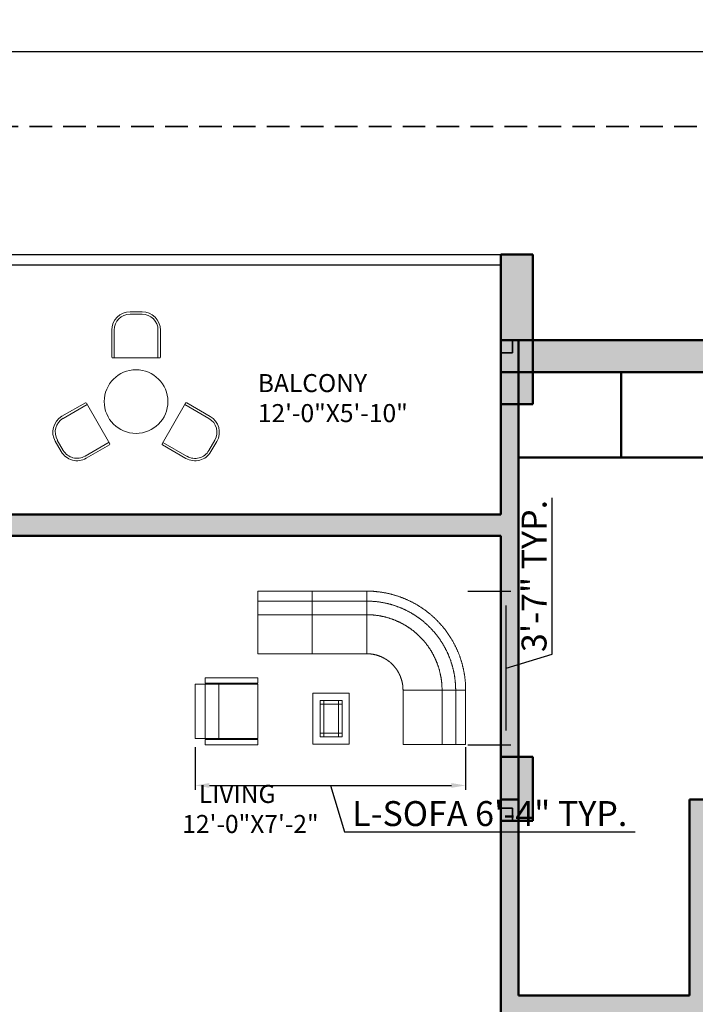
# Model space of a CAD drawing. Units: inches. Extents: x -7 to 1228, y -146 to 1091.
# Tile 87 of 88: x 816 to 1006, y 814 to 1091. Entities that reach past the tile are written whole.
import ezdxf

# ---------------------------------------------------------------- set-up
doc = ezdxf.new("R2010")
doc.units = ezdxf.units.IN
doc.linetypes.add('DASHED2', pattern=[9.525, 6.35, -3.175])
for name, color, linetype, lineweight in [('A-ANNO-DIMS', 2, 'Continuous', 18), ('A-AREA-IDEN', 7, 'Continuous', 18), ('A-COLS', 6, 'Continuous', 35), ('A-FURN', 8, 'Continuous', 18), ('A-GLAZ', 175, 'Continuous', 25), ('A-WALL', 7, 'Continuous', 50), ('A-WALL-PATT', 251, 'Continuous', 13), ('C-PROP', 1, 'DASHED2', 35)]:
    doc.layers.add(name, color=color, linetype=linetype, lineweight=lineweight)
doc.styles.get("Standard").update_dxf_attribs({"font": 'arial.ttf'})
doc.dimstyles.new('ISO-25', dxfattribs={"dimtxt": 7, "dimasz": 4, "dimexe": 1.25, "dimexo": 0.625, "dimtad": 1, "dimdec": 1, "dimlunit": 3, "dimtxsty": 'Standard', "dimcen": 2.5, "dimadec": 0, "dimazin": 0, "dimtfac": 1, "dimtdec": 1, "dimtmove": 1, "dimatfit": 3, "dimfxl": 1, "dimarcsym": 0})

# ---------------------------------------------------------------- blocks, each defined once
blk = doc.blocks.new('A$C5EBD0AE0')
for points in [[(1613, 2118, -75), (863, 2118, -75)], [(863, 2118, -75), (863, 1980, -75)], [(1613, 1255, -75), (1613, 2118, -75)], [(2363, 2118, -75), (1613, 2118, -75)], [(1613, 2118, -75), (1613, 1980, -75)], [(2363, 2118, -75), (2371, 2118, -75), (2379, 2118, -75), (2388, 2117, -75), (2396, 2117, -75), (2404, 2117, -75), (2413, 2117, -75), (2421, 2116, -75), (2429, 2116, -75), (2438, 2116, -75), (2446, 2115, -75), (2455, 2115, -75), (2463, 2114, -75), (2471, 2113, -75), (2480, 2113, -75), (2488, 2112, -75), (2496, 2111, -75), (2504, 2110, -75), (2513, 2109, -75), (2521, 2108, -75), (2529, 2107, -75), (2538, 2106, -75), (2546, 2105, -75), (2554, 2104, -75), (2563, 2103, -75), (2571, 2102, -75), (2579, 2100, -75), (2587, 2099, -75), (2596, 2098, -75), (2604, 2096, -75), (2612, 2095, -75), (2620, 2093, -75), (2628, 2092, -75), (2637, 2090, -75), (2645, 2088, -75), (2653, 2086, -75), (2661, 2085, -75), (2669, 2083, -75), (2677, 2081, -75), (2686, 2079, -75), (2694, 2077, -75), (2702, 2075, -75), (2710, 2073, -75), (2718, 2071, -75), (2726, 2068, -75), (2734, 2066, -75), (2742, 2064, -75), (2750, 2061, -75), (2758, 2059, -75), (2766, 2057, -75), (2774, 2054, -75), (2782, 2052, -75), (2790, 2049, -75), (2798, 2046, -75), (2806, 2044, -75), (2814, 2041, -75), (2822, 2038, -75), (2829, 2035, -75), (2837, 2032, -75), (2845, 2029, -75), (2853, 2026, -75), (2861, 2023, -75), (2869, 2020, -75), (2876, 2017, -75), (2884, 2014, -75), (2892, 2011, -75), (2899, 2008, -75), (2907, 2004, -75), (2915, 2001, -75), (2922, 1997, -75), (2930, 1994, -75), (2938, 1990, -75), (2945, 1987, -75), (2953, 1983, -75), (2960, 1980, -75), (2968, 1976, -75), (2975, 1972, -75), (2983, 1968, -75), (2990, 1965, -75), (2998, 1961, -75), (3005, 1957, -75), (3012, 1953, -75), (3020, 1949, -75), (3027, 1945, -75), (3034, 1941, -75), (3041, 1937, -75), (3049, 1932, -75), (3056, 1928, -75), (3063, 1924, -75), (3070, 1920, -75), (3077, 1915, -75), (3084, 1911, -75), (3092, 1906, -75), (3099, 1902, -75), (3106, 1897, -75), (3113, 1893, -75), (3120, 1888, -75), (3127, 1883, -75), (3133, 1879, -75), (3140, 1874, -75), (3147, 1869, -75), (3154, 1864, -75), (3161, 1859, -75), (3168, 1855, -75), (3174, 1850, -75), (3181, 1845, -75), (3188, 1840, -75), (3194, 1834, -75), (3201, 1829, -75), (3207, 1824, -75), (3214, 1819, -75), (3220, 1814, -75), (3227, 1808, -75), (3233, 1803, -75), (3240, 1798, -75), (3246, 1792, -75), (3253, 1787, -75), (3259, 1781, -75), (3265, 1776, -75), (3271, 1770, -75), (3278, 1765, -75), (3284, 1759, -75), (3290, 1753, -75), (3296, 1748, -75), (3302, 1742, -75), (3308, 1736, -75), (3314, 1730, -75), (3320, 1725, -75), (3326, 1719, -75), (3332, 1713, -75), (3338, 1707, -75), (3344, 1701, -75), (3349, 1695, -75), (3355, 1689, -75), (3361, 1683, -75), (3367, 1676, -75), (3372, 1670, -75), (3378, 1664, -75), (3383, 1658, -75), (3389, 1651, -75), (3394, 1645, -75), (3400, 1639, -75), (3405, 1632, -75), (3411, 1626, -75), (3416, 1620, -75), (3421, 1613, -75), (3426, 1607, -75), (3432, 1600, -75), (3437, 1593, -75), (3442, 1587, -75), (3447, 1580, -75), (3452, 1574, -75), (3457, 1567, -75), (3462, 1560, -75), (3467, 1553, -75), (3472, 1547, -75), (3477, 1540, -75), (3481, 1533, -75), (3486, 1526, -75), (3491, 1519, -75), (3495, 1512, -75), (3500, 1505, -75), (3505, 1498, -75), (3509, 1491, -75), (3514, 1484, -75), (3518, 1477, -75), (3523, 1470, -75), (3527, 1463, -75), (3531, 1456, -75), (3536, 1448, -75), (3540, 1441, -75), (3544, 1434, -75), (3548, 1427, -75), (3552, 1419, -75), (3556, 1412, -75), (3560, 1405, -75), (3564, 1397, -75), (3568, 1390, -75), (3572, 1383, -75), (3576, 1375, -75), (3580, 1368, -75), (3583, 1360, -75), (3587, 1353, -75), (3591, 1345, -75), (3594, 1338, -75), (3598, 1330, -75), (3601, 1323, -75), (3605, 1315, -75), (3608, 1307, -75), (3612, 1300, -75), (3615, 1292, -75), (3618, 1284, -75), (3621, 1277, -75), (3625, 1269, -75), (3628, 1261, -75), (3631, 1253, -75), (3634, 1246, -75), (3637, 1238, -75), (3640, 1230, -75), (3643, 1222, -75), (3645, 1214, -75), (3648, 1206, -75), (3651, 1198, -75), (3654, 1191, -75), (3656, 1183, -75), (3659, 1175, -75), (3661, 1167, -75), (3664, 1159, -75), (3666, 1151, -75), (3669, 1143, -75), (3671, 1135, -75), (3674, 1127, -75), (3676, 1119, -75), (3678, 1111, -75), (3680, 1102, -75), (3682, 1094, -75), (3684, 1086, -75), (3686, 1078, -75), (3688, 1070, -75), (3690, 1062, -75), (3692, 1054, -75), (3694, 1046, -75), (3696, 1037, -75), (3697, 1029, -75), (3699, 1021, -75), (3701, 1013, -75), (3702, 1005, -75), (3704, 996, -75), (3705, 988, -75), (3706, 980, -75), (3708, 972, -75), (3709, 963, -75), (3710, 955, -75), (3712, 947, -75), (3713, 939, -75), (3714, 930, -75), (3715, 922, -75), (3716, 914, -75), (3717, 905, -75), (3718, 897, -75), (3719, 889, -75), (3719, 880, -75), (3720, 872, -75), (3721, 864, -75), (3721, 855, -75), (3722, 847, -75), (3723, 839, -75), (3723, 830, -75), (3723, 822, -75), (3724, 814, -75), (3724, 805, -75), (3724, 797, -75), (3725, 789, -75), (3725, 780, -75), (3725, 772, -75), (3725, 764, -75), (3725, 755, -75)], [(2363, 1255, -75), (2363, 2118, -75)], [(2363, 1255, -75), (2363, 2118, -75)], [(863, 1980, -75), (1613, 1980, -75)], [(863, 1980, -75), (863, 1793, -75)], [(1613, 1980, -75), (2363, 1980, -75)], [(1613, 1980, -75), (1613, 1793, -75)], [(2363, 1980, -75), (2370, 1980, -75), (2378, 1980, -75), (2385, 1980, -75), (2393, 1980, -75), (2400, 1980, -75), (2408, 1979, -75), (2415, 1979, -75), (2423, 1979, -75), (2430, 1978, -75), (2438, 1978, -75), (2445, 1977, -75), (2453, 1977, -75), (2460, 1976, -75), (2468, 1976, -75), (2475, 1975, -75), (2483, 1974, -75), (2490, 1974, -75), (2498, 1973, -75), (2505, 1972, -75), (2513, 1971, -75), (2520, 1970, -75), (2527, 1969, -75), (2535, 1968, -75), (2542, 1967, -75), (2550, 1966, -75), (2557, 1965, -75), (2565, 1963, -75), (2572, 1962, -75), (2579, 1961, -75), (2587, 1960, -75), (2594, 1958, -75), (2602, 1957, -75), (2609, 1955, -75), (2616, 1954, -75), (2624, 1952, -75), (2631, 1950, -75), (2638, 1949, -75), (2646, 1947, -75), (2653, 1945, -75), (2660, 1943, -75), (2668, 1942, -75), (2675, 1940, -75), (2682, 1938, -75), (2689, 1936, -75), (2697, 1934, -75), (2704, 1932, -75), (2711, 1930, -75), (2718, 1927, -75), (2725, 1925, -75), (2733, 1923, -75), (2740, 1921, -75), (2747, 1918, -75), (2754, 1916, -75), (2761, 1914, -75), (2768, 1911, -75), (2775, 1909, -75), (2782, 1906, -75), (2789, 1903, -75), (2796, 1901, -75), (2803, 1898, -75), (2810, 1895, -75), (2817, 1893, -75), (2824, 1890, -75), (2831, 1887, -75), (2838, 1884, -75), (2845, 1881, -75), (2852, 1878, -75), (2859, 1875, -75), (2866, 1872, -75), (2873, 1869, -75), (2880, 1866, -75), (2886, 1863, -75), (2893, 1859, -75), (2900, 1856, -75), (2907, 1853, -75), (2913, 1849, -75), (2920, 1846, -75), (2927, 1843, -75), (2933, 1839, -75), (2940, 1836, -75), (2947, 1832, -75), (2953, 1828, -75), (2960, 1825, -75), (2966, 1821, -75), (2973, 1817, -75), (2979, 1814, -75), (2986, 1810, -75), (2992, 1806, -75), (2999, 1802, -75), (3005, 1798, -75), (3012, 1794, -75), (3018, 1790, -75), (3024, 1786, -75), (3031, 1782, -75), (3037, 1778, -75), (3043, 1774, -75), (3049, 1770, -75), (3056, 1765, -75), (3062, 1761, -75), (3068, 1757, -75), (3074, 1752, -75), (3080, 1748, -75), (3086, 1744, -75), (3092, 1739, -75), (3098, 1735, -75), (3104, 1730, -75), (3110, 1726, -75), (3116, 1721, -75), (3122, 1716, -75), (3128, 1712, -75), (3134, 1707, -75), (3140, 1702, -75), (3146, 1697, -75), (3151, 1693, -75), (3157, 1688, -75), (3163, 1683, -75), (3168, 1678, -75), (3174, 1673, -75), (3180, 1668, -75), (3185, 1663, -75), (3191, 1658, -75), (3196, 1653, -75), (3202, 1648, -75), (3207, 1642, -75), (3213, 1637, -75), (3218, 1632, -75), (3223, 1627, -75), (3229, 1621, -75), (3234, 1616, -75), (3239, 1611, -75), (3245, 1605, -75), (3250, 1600, -75), (3255, 1594, -75), (3260, 1589, -75), (3265, 1583, -75), (3270, 1578, -75), (3275, 1572, -75), (3280, 1567, -75), (3285, 1561, -75), (3290, 1555, -75), (3295, 1550, -75), (3300, 1544, -75), (3305, 1538, -75), (3310, 1532, -75), (3314, 1527, -75), (3319, 1521, -75), (3324, 1515, -75), (3328, 1509, -75), (3333, 1503, -75), (3338, 1497, -75), (3342, 1491, -75), (3347, 1485, -75), (3351, 1479, -75), (3355, 1473, -75), (3360, 1467, -75), (3364, 1461, -75), (3368, 1454, -75), (3373, 1448, -75), (3377, 1442, -75), (3381, 1436, -75), (3385, 1430, -75), (3389, 1423, -75), (3394, 1417, -75), (3398, 1411, -75), (3402, 1404, -75), (3406, 1398, -75), (3409, 1391, -75), (3413, 1385, -75), (3417, 1379, -75), (3421, 1372, -75), (3425, 1366, -75), (3428, 1359, -75), (3432, 1352, -75), (3436, 1346, -75), (3439, 1339, -75), (3443, 1333, -75), (3446, 1326, -75), (3450, 1319, -75), (3453, 1313, -75), (3457, 1306, -75), (3460, 1299, -75), (3463, 1293, -75), (3467, 1286, -75), (3470, 1279, -75), (3473, 1272, -75), (3476, 1265, -75), (3479, 1258, -75), (3483, 1252, -75), (3486, 1245, -75), (3489, 1238, -75), (3491, 1231, -75), (3494, 1224, -75), (3497, 1217, -75), (3500, 1210, -75), (3503, 1203, -75), (3506, 1196, -75), (3508, 1189, -75), (3511, 1182, -75), (3513, 1175, -75), (3516, 1168, -75), (3519, 1161, -75), (3521, 1154, -75), (3523, 1147, -75), (3526, 1139, -75), (3528, 1132, -75), (3530, 1125, -75), (3533, 1118, -75), (3535, 1111, -75), (3537, 1104, -75), (3539, 1096, -75), (3541, 1089, -75), (3543, 1082, -75), (3545, 1075, -75), (3547, 1067, -75), (3549, 1060, -75), (3551, 1053, -75), (3553, 1046, -75), (3554, 1038, -75), (3556, 1031, -75), (3558, 1024, -75), (3559, 1016, -75), (3561, 1009, -75), (3563, 1002, -75), (3564, 994, -75), (3566, 987, -75), (3567, 979, -75), (3568, 972, -75), (3570, 965, -75), (3571, 957, -75), (3572, 950, -75), (3573, 942, -75), (3574, 935, -75), (3575, 928, -75), (3576, 920, -75), (3577, 913, -75), (3578, 905, -75), (3579, 898, -75), (3580, 890, -75), (3581, 883, -75), (3582, 875, -75), (3582, 868, -75), (3583, 860, -75), (3584, 853, -75), (3584, 845, -75), (3585, 838, -75), (3585, 830, -75), (3586, 823, -75), (3586, 815, -75), (3586, 808, -75), (3587, 800, -75), (3587, 793, -75), (3587, 785, -75), (3587, 778, -75), (3588, 770, -75), (3588, 763, -75), (3588, 755, -75)], [(863, 1793, -75), (1613, 1793, -75)], [(863, 1793, -75), (863, 1255, -75)], [(1613, 1793, -75), (1613, 1255, -75)], [(1613, 1793, -75), (2363, 1793, -75)], [(2363, 1793, -75), (2369, 1793, -75), (2375, 1793, -75), (2382, 1793, -75), (2388, 1792, -75), (2394, 1792, -75), (2401, 1792, -75), (2407, 1792, -75), (2414, 1791, -75), (2420, 1791, -75), (2426, 1791, -75), (2433, 1790, -75), (2439, 1790, -75), (2445, 1789, -75), (2452, 1789, -75), (2458, 1788, -75), (2464, 1788, -75), (2471, 1787, -75), (2477, 1786, -75), (2483, 1786, -75), (2490, 1785, -75), (2496, 1784, -75), (2502, 1783, -75), (2509, 1782, -75), (2515, 1781, -75), (2521, 1781, -75), (2527, 1780, -75), (2534, 1779, -75), (2540, 1777, -75), (2546, 1776, -75), (2553, 1775, -75), (2559, 1774, -75), (2565, 1773, -75), (2571, 1772, -75), (2577, 1770, -75), (2584, 1769, -75), (2590, 1768, -75), (2596, 1766, -75), (2602, 1765, -75), (2609, 1763, -75), (2615, 1762, -75), (2621, 1760, -75), (2627, 1758, -75), (2633, 1757, -75), (2639, 1755, -75), (2645, 1753, -75), (2652, 1752, -75), (2658, 1750, -75), (2664, 1748, -75), (2670, 1746, -75), (2676, 1744, -75), (2682, 1742, -75), (2688, 1740, -75), (2694, 1738, -75), (2700, 1736, -75), (2706, 1734, -75), (2712, 1732, -75), (2718, 1730, -75), (2724, 1728, -75), (2730, 1725, -75), (2736, 1723, -75), (2742, 1721, -75), (2748, 1719, -75), (2754, 1716, -75), (2760, 1714, -75), (2766, 1711, -75), (2771, 1709, -75), (2777, 1706, -75), (2783, 1704, -75), (2789, 1701, -75), (2795, 1698, -75), (2800, 1696, -75), (2806, 1693, -75), (2812, 1690, -75), (2818, 1688, -75), (2823, 1685, -75), (2829, 1682, -75), (2835, 1679, -75), (2840, 1676, -75), (2846, 1673, -75), (2852, 1670, -75), (2857, 1667, -75), (2863, 1664, -75), (2868, 1661, -75), (2874, 1658, -75), (2880, 1655, -75), (2885, 1652, -75), (2891, 1648, -75), (2896, 1645, -75), (2901, 1642, -75), (2907, 1638, -75), (2912, 1635, -75), (2918, 1632, -75), (2923, 1628, -75), (2928, 1625, -75), (2934, 1621, -75), (2939, 1618, -75), (2944, 1614, -75), (2950, 1611, -75), (2955, 1607, -75), (2960, 1603, -75), (2965, 1600, -75), (2970, 1596, -75), (2976, 1592, -75), (2981, 1589, -75), (2986, 1585, -75), (2991, 1581, -75), (2996, 1577, -75), (3001, 1573, -75), (3006, 1569, -75), (3011, 1565, -75), (3016, 1561, -75), (3021, 1557, -75), (3026, 1553, -75), (3031, 1549, -75), (3035, 1545, -75), (3040, 1541, -75), (3045, 1537, -75), (3050, 1532, -75), (3055, 1528, -75), (3059, 1524, -75), (3064, 1520, -75), (3069, 1515, -75), (3073, 1511, -75), (3078, 1507, -75), (3083, 1502, -75), (3087, 1498, -75), (3092, 1493, -75), (3096, 1489, -75), (3101, 1484, -75), (3105, 1480, -75), (3110, 1475, -75), (3114, 1471, -75), (3118, 1466, -75), (3123, 1461, -75), (3127, 1457, -75), (3131, 1452, -75), (3136, 1447, -75), (3140, 1442, -75), (3144, 1438, -75), (3148, 1433, -75), (3152, 1428, -75), (3156, 1423, -75), (3161, 1418, -75), (3165, 1413, -75), (3169, 1408, -75), (3173, 1404, -75), (3177, 1399, -75), (3181, 1394, -75), (3184, 1388, -75), (3188, 1383, -75), (3192, 1378, -75), (3196, 1373, -75), (3200, 1368, -75), (3203, 1363, -75), (3207, 1358, -75), (3211, 1353, -75), (3215, 1347, -75), (3218, 1342, -75), (3222, 1337, -75), (3225, 1332, -75), (3229, 1326, -75), (3232, 1321, -75), (3236, 1316, -75), (3239, 1310, -75), (3243, 1305, -75), (3246, 1299, -75), (3249, 1294, -75), (3253, 1289, -75), (3256, 1283, -75), (3259, 1278, -75), (3262, 1272, -75), (3265, 1267, -75), (3268, 1261, -75), (3272, 1255, -75), (3275, 1250, -75), (3278, 1244, -75), (3281, 1239, -75), (3284, 1233, -75), (3286, 1227, -75), (3289, 1222, -75), (3292, 1216, -75), (3295, 1210, -75), (3298, 1205, -75), (3300, 1199, -75), (3303, 1193, -75), (3306, 1187, -75), (3309, 1181, -75), (3311, 1176, -75), (3314, 1170, -75), (3316, 1164, -75), (3319, 1158, -75), (3321, 1152, -75), (3324, 1146, -75), (3326, 1140, -75), (3328, 1135, -75), (3331, 1129, -75), (3333, 1123, -75), (3335, 1117, -75), (3337, 1111, -75), (3339, 1105, -75), (3342, 1099, -75), (3344, 1093, -75), (3346, 1087, -75), (3348, 1081, -75), (3350, 1075, -75), (3352, 1069, -75), (3354, 1062, -75), (3355, 1056, -75), (3357, 1050, -75), (3359, 1044, -75), (3361, 1038, -75), (3363, 1032, -75), (3364, 1026, -75), (3366, 1020, -75), (3367, 1013, -75), (3369, 1007, -75), (3371, 1001, -75), (3372, 995, -75), (3373, 989, -75), (3375, 983, -75), (3376, 976, -75), (3378, 970, -75), (3379, 964, -75), (3380, 958, -75), (3381, 951, -75), (3383, 945, -75), (3384, 939, -75), (3385, 933, -75), (3386, 926, -75), (3387, 920, -75), (3388, 914, -75), (3389, 907, -75), (3390, 901, -75), (3391, 895, -75), (3392, 889, -75), (3392, 882, -75), (3393, 876, -75), (3394, 870, -75), (3394, 863, -75), (3395, 857, -75), (3396, 851, -75), (3396, 844, -75), (3397, 838, -75), (3397, 832, -75), (3398, 825, -75), (3398, 819, -75), (3399, 812, -75), (3399, 806, -75), (3399, 800, -75), (3399, 793, -75), (3400, 787, -75), (3400, 781, -75), (3400, 774, -75), (3400, 768, -75), (3400, 762, -75), (3400, 755, -75)], [(863, 1255, -75), (1613, 1255, -75)], [(1613, 1255, -75), (2363, 1255, -75)], [(2363, 1255, -75), (2366, 1255, -75), (2369, 1255, -75), (2372, 1255, -75), (2375, 1255, -75), (2378, 1255, -75), (2381, 1255, -75), (2384, 1255, -75), (2387, 1255, -75), (2390, 1254, -75), (2393, 1254, -75), (2396, 1254, -75), (2399, 1254, -75), (2402, 1254, -75), (2406, 1253, -75), (2409, 1253, -75), (2412, 1253, -75), (2415, 1252, -75), (2418, 1252, -75), (2421, 1252, -75), (2424, 1251, -75), (2427, 1251, -75), (2430, 1251, -75), (2433, 1250, -75), (2436, 1250, -75), (2439, 1249, -75), (2442, 1249, -75), (2445, 1248, -75), (2448, 1248, -75), (2451, 1247, -75), (2454, 1247, -75), (2457, 1246, -75), (2460, 1246, -75), (2463, 1245, -75), (2466, 1244, -75), (2469, 1244, -75), (2472, 1243, -75), (2475, 1242, -75), (2478, 1242, -75), (2481, 1241, -75), (2484, 1240, -75), (2487, 1239, -75), (2490, 1239, -75), (2493, 1238, -75), (2496, 1237, -75), (2499, 1236, -75), (2502, 1235, -75), (2505, 1235, -75), (2508, 1234, -75), (2511, 1233, -75), (2514, 1232, -75), (2517, 1231, -75), (2519, 1230, -75), (2522, 1229, -75), (2525, 1228, -75), (2528, 1227, -75), (2531, 1226, -75), (2534, 1225, -75), (2537, 1224, -75), (2540, 1223, -75), (2543, 1222, -75), (2545, 1221, -75), (2548, 1219, -75), (2551, 1218, -75), (2554, 1217, -75), (2557, 1216, -75), (2560, 1215, -75), (2562, 1214, -75), (2565, 1212, -75), (2568, 1211, -75), (2571, 1210, -75), (2574, 1209, -75), (2576, 1207, -75), (2579, 1206, -75), (2582, 1205, -75), (2585, 1203, -75), (2587, 1202, -75), (2590, 1200, -75), (2593, 1199, -75), (2596, 1198, -75), (2598, 1196, -75), (2601, 1195, -75), (2604, 1193, -75), (2606, 1192, -75), (2609, 1190, -75), (2612, 1189, -75), (2614, 1187, -75), (2617, 1186, -75), (2620, 1184, -75), (2622, 1182, -75), (2625, 1181, -75), (2628, 1179, -75), (2630, 1178, -75), (2633, 1176, -75), (2635, 1174, -75), (2638, 1173, -75), (2640, 1171, -75), (2643, 1169, -75), (2645, 1168, -75), (2648, 1166, -75), (2651, 1164, -75), (2653, 1162, -75), (2656, 1160, -75), (2658, 1159, -75), (2660, 1157, -75), (2663, 1155, -75), (2665, 1153, -75), (2668, 1151, -75), (2670, 1149, -75), (2673, 1147, -75), (2675, 1146, -75), (2677, 1144, -75), (2680, 1142, -75), (2682, 1140, -75), (2685, 1138, -75), (2687, 1136, -75), (2689, 1134, -75), (2692, 1132, -75), (2694, 1130, -75), (2696, 1128, -75), (2698, 1126, -75), (2701, 1124, -75), (2703, 1122, -75), (2705, 1119, -75), (2707, 1117, -75), (2710, 1115, -75), (2712, 1113, -75), (2714, 1111, -75), (2716, 1109, -75), (2718, 1107, -75), (2720, 1104, -75), (2723, 1102, -75), (2725, 1100, -75), (2727, 1098, -75), (2729, 1096, -75), (2731, 1093, -75), (2733, 1091, -75), (2735, 1089, -75), (2737, 1086, -75), (2739, 1084, -75), (2741, 1082, -75), (2743, 1079, -75), (2745, 1077, -75), (2747, 1075, -75), (2749, 1072, -75), (2751, 1070, -75), (2753, 1068, -75), (2755, 1065, -75), (2757, 1063, -75), (2759, 1060, -75), (2761, 1058, -75), (2762, 1056, -75), (2764, 1053, -75), (2766, 1051, -75), (2768, 1048, -75), (2770, 1046, -75), (2771, 1043, -75), (2773, 1041, -75), (2775, 1038, -75), (2777, 1036, -75), (2778, 1033, -75), (2780, 1030, -75), (2782, 1028, -75), (2783, 1025, -75), (2785, 1023, -75), (2787, 1020, -75), (2788, 1018, -75), (2790, 1015, -75), (2791, 1012, -75), (2793, 1010, -75), (2795, 1007, -75), (2796, 1004, -75), (2798, 1002, -75), (2799, 999, -75), (2801, 996, -75), (2802, 994, -75), (2804, 991, -75), (2805, 988, -75), (2806, 985, -75), (2808, 983, -75), (2809, 980, -75), (2811, 977, -75), (2812, 975, -75), (2813, 972, -75), (2815, 969, -75), (2816, 966, -75), (2817, 963, -75), (2818, 961, -75), (2820, 958, -75), (2821, 955, -75), (2822, 952, -75), (2823, 949, -75), (2825, 947, -75), (2826, 944, -75), (2827, 941, -75), (2828, 938, -75), (2829, 935, -75), (2830, 932, -75), (2831, 929, -75), (2832, 927, -75), (2833, 924, -75), (2834, 921, -75), (2835, 918, -75), (2836, 915, -75), (2837, 912, -75), (2838, 909, -75), (2839, 906, -75), (2840, 903, -75), (2841, 900, -75), (2842, 897, -75), (2843, 894, -75), (2844, 892, -75), (2844, 889, -75), (2845, 886, -75), (2846, 883, -75), (2847, 880, -75), (2848, 877, -75), (2848, 874, -75), (2849, 871, -75), (2850, 868, -75), (2850, 865, -75), (2851, 862, -75), (2852, 859, -75), (2852, 856, -75), (2853, 853, -75), (2854, 850, -75), (2854, 847, -75), (2855, 844, -75), (2855, 841, -75), (2856, 838, -75), (2856, 835, -75), (2857, 832, -75), (2857, 829, -75), (2858, 826, -75), (2858, 822, -75), (2858, 819, -75), (2859, 816, -75), (2859, 813, -75), (2860, 810, -75), (2860, 807, -75), (2860, 804, -75), (2860, 801, -75), (2861, 798, -75), (2861, 795, -75), (2861, 792, -75), (2861, 789, -75), (2862, 786, -75), (2862, 783, -75), (2862, 780, -75), (2862, 777, -75), (2862, 774, -75), (2862, 771, -75), (2862, 767, -75), (2863, 764, -75), (2863, 761, -75), (2863, 758, -75), (2863, 755, -75)], [(0, 837, -75), (0, 87, -75)], [(863, 837, -75), (0, 837, -75)], [(138, 925, -75), (863, 925, -75)], [(138, 850, -75), (138, 925, -75)], [(863, 850, -75), (138, 850, -75)], [(138, 87, -75), (138, 837, -75)], [(325, 87, -75), (325, 837, -75)], [(863, 925, -75), (863, 850, -75)], [(863, 87, -75), (863, 837, -75)], [(2863, 755, -75), (2863, 5, -75)], [(3400, 755, -75), (2863, 755, -75)], [(3400, 755, -75), (3400, 5, -75)], [(3588, 755, -75), (3400, 755, -75)], [(3588, 755, -75), (3588, 5, -75)], [(3725, 755, -75), (3588, 755, -75)], [(3725, 5, -75), (3725, 755, -75)], [(0, 87, -75), (138, 87, -75)], [(138, 87, -75), (325, 87, -75)], [(863, 75, -75), (138, 75, -75)], [(138, 75, -75), (138, 0, -75)], [(325, 87, -75), (863, 87, -75)], [(863, 0, -75), (863, 75, -75)], [(3400, 5, -75), (2863, 5, -75)], [(2863, 5, -75), (3725, 5, -75)], [(3588, 5, -75), (3400, 5, -75)], [(3725, 5, -75), (3588, 5, -75)], [(138, 0, -75), (863, 0, -75)]]:
    blk.add_polyline3d(points)
for points in [[(1623, 10), (1623, 710), (1623, 710, 25), (1623, 10, 25)], [(1623, 710), (2123, 710), (2123, 710, 25), (1623, 710, 25)], [(2123, 710), (2123, 10), (2123, 10, 25), (2123, 710, 25)], [(1723, 610, -675), (1773, 610, -675), (1773, 610), (1723, 610)], [(1773, 610, -675), (1723, 610, -675), (1723, 610), (1773, 610)], [(1723, 610, -675), (1723, 560, -675), (1723, 560), (1723, 610)], [(1723, 560, -675), (1773, 560, -675), (1773, 560), (1723, 560)], [(1723, 560, -375), (1723, 160, -375), (1723, 160, -350), (1723, 560, -350)], [(1773, 610, -675), (1773, 560, -675), (1773, 560), (1773, 610)], [(1773, 560, -675), (1773, 610, -675), (1773, 610), (1773, 560)], [(1973, 610, -375), (1773, 610, -375), (1773, 610, -350), (1973, 610, -350)], [(2023, 560, -375), (1773, 560, -375), (1773, 560, -350), (2023, 560, -350)], [(1773, 560, -375), (1773, 110, -375), (1773, 110, -350), (1773, 560, -350)], [(2023, 610, -675), (1973, 610, -675), (1973, 610), (2023, 610)], [(1973, 610, -675), (1973, 560, -675), (1973, 560), (1973, 610)], [(1973, 110, -375), (1973, 610, -375), (1973, 610, -350), (1973, 110, -350)], [(1973, 560, -675), (2023, 560, -675), (2023, 560), (1973, 560)], [(2023, 560, -675), (2023, 610, -675), (2023, 610), (2023, 560)], [(2023, 160, -375), (2023, 560, -375), (2023, 560, -350), (2023, 160, -350)], [(1723, 110, -675), (1723, 160, -675), (1723, 160), (1723, 110)], [(1723, 160, -675), (1773, 160, -675), (1773, 160), (1723, 160)], [(1723, 160, -375), (2023, 160, -375), (2023, 160, -350), (1723, 160, -350)], [(1773, 160, -675), (1773, 110, -675), (1773, 110), (1773, 160)], [(1973, 110, -675), (1973, 160, -675), (1973, 160), (1973, 110)], [(1973, 160, -675), (2023, 160, -675), (2023, 160), (1973, 160)], [(2023, 110, -675), (2023, 160, -675), (2023, 160), (2023, 110)], [(2123, 10), (1623, 10), (1623, 10, 25), (2123, 10, 25)], [(1773, 110, -675), (1723, 110, -675), (1723, 110), (1773, 110)], [(1773, 110, -375), (1973, 110, -375), (1973, 110, -350), (1773, 110, -350)], [(2023, 110, -675), (1973, 110, -675), (1973, 110), (2023, 110)]]:
    blk.add_3dface(points)
blk = doc.blocks.new('*D11')
at = {"layer": 'A-ANNO-DIMS', "color": 0, "lineweight": -2, "transparency": 16777216}
for p, q in [((0, 1061.62), (0, 1083.25)), ((4, 1082), (1183, 1082)), ((1187, 1061.62), (1187, 1083.25))]:
    blk.add_line(p, q, dxfattribs=at)
at = {"layer": 'A-ANNO-DIMS', "color": 0, "transparency": 16777216}
for points in [[(4, 1082.67), (4, 1081.33), (0, 1082)], [(1183, 1082.67), (1183, 1081.33), (1187, 1082)]]:
    blk.add_solid(points, dxfattribs=at)
at = {"layer": 'Defpoints', "color": 0, "transparency": 16777216}
for p in [(1187, 1082), (0, 1061), (1187, 1061)]:
    blk.add_point(p, dxfattribs=at)
at = {"layer": 'A-ANNO-DIMS', "color": 0, "transparency": 16777216, "insert": (593.5, 1086.2), "char_height": 7, "attachment_point": 5}
blk.add_mtext('98\'-11"', dxfattribs=at)
blk = doc.blocks.new('A$C670C3AF2')
for p, q in [((1122, 1874), (972, 1874)), ((1122, 1844), (972, 1844)), ((742, 1644), (742, 1304)), ((772, 1644), (772, 1294)), ((1322, 1294), (1322, 1644)), ((1352, 1304), (1352, 1644)), ((752, 1294), (1342, 1294)), ((409, 730), (115, 560)), ((433, 709), (130, 534)), ((718, 215), (423, 726)), ((1669, 725), (1374, 214)), ((1963, 533), (1659, 708)), ((1978, 559), (1683, 729)), ((56, 261), (131, 131)), ((1961, 130), (2036, 259)), ((30, 246), (105, 116)), ((405, 58), (708, 233)), ((420, 32), (714, 202)), ((1378, 200), (1673, 30)), ((1384, 231), (1688, 56)), ((1987, 115), (2062, 244))]:
    blk.add_line(p, q)
blk.add_circle((1046, 745), 400)
for centre, radius, start, end in [((972, 1644), 230, 90, 180), ((1122, 1644), 230, 0, 90), ((972, 1644), 200, 90, 180), ((1122, 1644), 200, 0, 90), ((752, 1304), 10, 180, 270), ((1342, 1304), 10, 270, 0), ((414, 721), 10, 30, 120), ((1678, 720), 10, 60, 150), ((230, 361), 230, 120, 210), ((230, 361), 200, 120, 210), ((1863, 359), 200, 330, 60), ((1863, 359), 230, 330, 60), ((305, 231), 200, 210, 300), ((709, 210), 10, 300, 30), ((1383, 209), 10, 150, 240), ((1788, 230), 200, 240, 330), ((305, 231), 230, 210, 300), ((1788, 230), 230, 240, 330)]:
    blk.add_arc(centre, radius, start, end)
blk = doc.blocks.new('*D42')
at = {"layer": 'A-ANNO-DIMS', "color": 0, "lineweight": -2, "transparency": 16777216}
for p, q in [((865.21, 886.72), (865.21, 874.71)), ((941.15, 886.72), (941.15, 874.71)), ((869.21, 875.96), (937.15, 875.96)), ((903.18, 875.96), (907.1, 862.9)), ((907.1, 862.9), (988.74, 862.9))]:
    blk.add_line(p, q, dxfattribs=at)
at = {"layer": 'A-ANNO-DIMS', "color": 0, "transparency": 16777216}
for points in [[(869.21, 876.62), (869.21, 875.29), (865.21, 875.96)], [(937.15, 876.62), (937.15, 875.29), (941.15, 875.96)]]:
    blk.add_solid(points, dxfattribs=at)
at = {"layer": 'Defpoints', "color": 0, "transparency": 16777216}
for p in [(865.21, 887.35), (941.15, 887.35), (941.15, 875.96)]:
    blk.add_point(p, dxfattribs=at)
at = {"layer": 'A-ANNO-DIMS', "color": 0, "transparency": 16777216, "insert": (947.92, 867.15), "char_height": 7, "attachment_point": 5}
blk.add_mtext('L-SOFA 6\'-4" TYP.', dxfattribs=at)
blk = doc.blocks.new('*D43')
at = {"layer": 'A-ANNO-DIMS', "color": 0, "lineweight": -2, "transparency": 16777216}
for p, q in [((965.46, 912.81), (965.46, 956.72)), ((941.77, 930.52), (953.79, 930.52)), ((952.54, 891.35), (952.54, 926.52)), ((952.54, 908.93), (965.46, 912.81)), ((941.77, 887.35), (953.79, 887.35))]:
    blk.add_line(p, q, dxfattribs=at)
at = {"layer": 'A-ANNO-DIMS', "color": 0, "transparency": 16777216}
for points in [[(951.87, 926.52), (953.21, 926.52), (952.54, 930.52)], [(951.87, 891.35), (953.21, 891.35), (952.54, 887.35)]]:
    blk.add_solid(points, dxfattribs=at)
at = {"layer": 'Defpoints', "color": 0, "transparency": 16777216}
for p in [(941.15, 930.52), (952.54, 930.52), (941.15, 887.35)]:
    blk.add_point(p, dxfattribs=at)
at = {"layer": 'A-ANNO-DIMS', "color": 0, "transparency": 16777216, "insert": (961.25, 934.76), "char_height": 7, "attachment_point": 5, "rotation": 90}
blk.add_mtext('3\'-7" TYP.', dxfattribs=at)

msp = doc.modelspace()

# ---------------------------------------------------------------- hatches: boundary and pattern name
at = {"layer": 'A-COLS'}
h = msp.add_hatch(color=256, dxfattribs=at)
h.dxf.hatch_style = 1
h.paths.add_polyline_path([(951, 983), (960, 983), (960, 1001), (954.29, 1001), (954.29, 997.45), (951, 997.45)])
h = msp.add_hatch(color=256, dxfattribs=at)
h.dxf.hatch_style = 1
h.paths.add_polyline_path([(954.29, 997.45), (954.29, 1001), (951, 1001), (951, 997.45)])
h = msp.add_hatch(color=256, dxfattribs=at)
h.dxf.hatch_style = 1
h.paths.add_polyline_path([(960, 884), (951, 884), (951, 869.55), (954.29, 869.55), (954.29, 866), (960, 866)])
h = msp.add_hatch(color=256, dxfattribs=at)
h.dxf.hatch_style = 1
h.paths.add_polyline_path([(954.29, 869.55), (951, 869.55), (951, 866), (954.29, 866)])
at = {"layer": 'A-WALL-PATT'}
h = msp.add_hatch(color=256, dxfattribs=at)
h.dxf.hatch_style = 1
h.paths.add_polyline_path([(69, 568), (60, 568), (60, 493), (63.29, 493), (69, 493)])
h.paths.add_polyline_path([(69, 662.41), (60, 662.41), (60, 586), (69, 586)], flags=17)
h.paths.add_polyline_path([(69, 723), (184, 723), (184, 734), (179, 734), (179, 728), (69, 728), (69, 741.62), (60, 741.62), (60, 698.41), (69, 698.41)], flags=17)
h.paths.add_polyline_path([(69, 782), (231, 782), (231, 728), (231, 723), (231, 586), (236, 586), (236, 787), (69, 787), (69, 800.13), (60, 800.13), (60, 765.62), (69, 765.62)])
h.paths.add_polyline_path([(184, 842), (189, 842), (189, 848), (173, 848), (173, 842), (179, 842), (179, 787), (184, 787)])
h.paths.add_polyline_path([(118.22, 69), (69, 69), (69, 60), (118.22, 60)])
h.paths.add_polyline_path([(227, 69), (154.22, 69), (154.22, 60), (227, 60)])
h.paths.add_polyline_path([(236, 60), (232.71, 60), (227, 60), (227, 36), (236, 36)])
h.paths.add_polyline_path([(389, 60), (380, 60), (380, 36), (389, 36)])
h.paths.add_polyline_path([(384, 181), (380, 181), (380, 115), (380, 78), (384, 78)])
h.paths.add_polyline_path([(380, 115), (334.55, 115), (334.55, 109), (380, 109)])
h.paths.add_polyline_path([(274.55, 115), (236, 115), (236, 201), (232.71, 201), (231, 201), (231, 78), (236, 78), (236, 109), (274.55, 109)])
h.paths.add_polyline_path([(69, 123), (60, 123), (60, 78), (69, 78)])
h.paths.add_polyline_path([(69, 201), (60, 201), (60, 159), (69, 159)])
h.paths.add_polyline_path([(143, 219), (69, 219), (69, 213), (143, 213)], flags=17)
h.paths.add_polyline_path([(189, 219), (184, 219), (184, 274), (231, 274), (231, 219), (236, 219), (236, 279), (184, 279), (184, 297), (179, 297), (179, 279), (69, 279), (69, 290.91), (60, 290.91), (60, 262.18), (69, 262.18), (69, 274), (179, 274), (179, 219), (173, 219), (173, 213), (189, 213)])
h.paths.add_polyline_path([(69, 238.18), (60, 238.18), (60, 219), (69, 219)], flags=17)
h.paths.add_polyline_path([(69, 333), (60, 333), (60, 314.91), (69, 314.91), (69, 316.96)])
h.paths.add_polyline_path([(190, 338), (184, 338), (69, 338), (69, 333), (179, 333), (179, 327), (184, 327), (184, 333.02), (190, 333.05)])
h.paths.add_polyline_path([(69, 386.81), (60, 386.81), (60, 351), (69, 351)])
h.paths.add_polyline_path([(69, 475), (60, 475), (60, 422.81), (69, 422.81)])
h.paths.add_polyline_path([(236, 475), (231, 475), (231, 351.24), (236, 351.24)])
h.paths.add_polyline_path([(384, 475), (380, 475), (380, 362), (384, 362)])
h.paths.add_polyline_path([(547, 307), (439, 307), (439, 356), (445, 356), (445, 362), (433, 362), (433, 307), (380, 307), (380, 244), (380, 241), (384, 241), (384, 301), (433, 301), (433, 277), (439, 277), (439, 301), (547, 301)])
h.paths.add_polyline_path([(547, 241), (439, 241), (439, 247), (433, 247), (433, 235), (547, 235)])
h.paths.add_polyline_path([(450, 69), (440.29, 69), (424.89, 69), (389, 69), (389, 60), (450, 60)])
h.paths.add_polyline_path([(547, 69), (486, 69), (486, 60), (547, 60)])
h.paths.add_polyline_path([(556, 148.27), (547, 148.27), (547, 78), (556, 78)])
h.paths.add_polyline_path([(556, 223), (547, 223), (547, 195), (547, 184.27), (556, 184.27)])
h.paths.add_polyline_path([(556, 311.19), (547, 311.19), (547, 273.08), (556, 273.08)])
h.paths.add_polyline_path([(556, 344), (552.71, 344), (547, 344), (547, 335.19), (556, 335.19)])
h.paths.add_polyline_path([(556, 249.08), (547, 249.08), (547, 241), (556, 241)])
h.paths.add_polyline_path([(547, 362), (475, 362), (475, 356), (547, 356)], flags=0)
h.paths.add_polyline_path([(556, 399.62), (547, 399.62), (547, 362), (556, 362)])
h.paths.add_polyline_path([(556, 475), (547, 475), (547, 435.62), (556, 435.62)])
h.paths.add_polyline_path([(547, 493), (389, 493), (389, 487), (547, 487)])
h.paths.add_polyline_path([(380, 493), (278, 493), (278, 487), (380, 487)])
h.paths.add_polyline_path([(227, 493), (69, 493), (69, 487), (227, 487)])
h.paths.add_polyline_path([(643, 122.44), (634, 122.44), (634, 78), (643, 78)])
h.paths.add_polyline_path([(702.5, 69), (692.79, 69), (677.39, 69), (643, 69), (643, 60), (702.5, 60)])
h.paths.add_polyline_path([(798, 69), (738.5, 69), (738.5, 60), (798, 60)])
h.paths.add_polyline_path([(807, 60), (803.71, 60), (798, 60), (798, 36), (807, 36)])
h.paths.add_polyline_path([(807, 109), (846.75, 109), (846.75, 115), (807, 115), (807, 159), (802, 159), (802, 78), (807, 78)])
h.paths.add_polyline_path([(807, 201), (802, 201), (802, 195), (807, 195)])
h.paths.add_polyline_path([(643, 201), (634, 201), (634, 158.44), (643, 158.44)])
h.paths.add_polyline_path([(756, 225), (751, 225), (751, 219), (643, 219), (643, 213), (756, 213)])
h.paths.add_polyline_path([(643, 240.85), (634, 240.85), (634, 219), (643, 219)])
h.paths.add_polyline_path([(643, 274), (643, 288.63), (634, 288.63), (634, 264.85), (643, 264.85)])
h.paths.add_polyline_path([(802, 279), (756, 279), (756, 297), (751, 297), (751, 279), (643, 279), (643, 274), (751, 274), (751, 255), (756, 255), (756, 274), (802, 274)])
h.paths.add_polyline_path([(807, 333), (803.71, 333), (802, 333), (802, 279), (802, 274), (802, 219), (807, 219)])
h.paths.add_polyline_path([(956, 182), (951, 182), (951, 115), (906.75, 115), (906.75, 109), (951, 109), (951, 78), (956, 78)])
h.paths.add_polyline_path([(960, 60), (951, 60), (951, 36), (960, 36)])
h.paths.add_polyline_path([(1021, 69), (1005.78, 69), (960, 69), (960, 60), (1021, 60)])
h.paths.add_polyline_path([(956, 224), (951, 224), (951, 218), (956, 218)])
h.paths.add_polyline_path([(956, 302), (1004, 302), (1004, 278), (1010, 278), (1010, 302), (1118, 302), (1118, 290.81), (1127, 290.81), (1127, 326.97), (1118, 326.97), (1118, 320.97), (1118, 307), (1010, 307), (1010, 356), (1016, 356), (1016, 362), (1004, 362), (1004, 307), (951, 307), (951, 244), (951, 242), (954.29, 242), (956, 242)])
h.paths.add_polyline_path([(643, 333), (634, 333), (634, 312.63), (643, 312.63), (643, 316.96)])
h.paths.add_polyline_path([(756, 338), (643, 338), (643, 333), (751, 333), (751, 327), (756, 327)])
h.paths.add_polyline_path([(643, 388), (634, 388), (634, 351), (643, 351)])
h.paths.add_polyline_path([(807, 357), (802, 357), (802, 351), (807, 351)])
h.paths.add_polyline_path([(807, 475), (802, 475), (802, 393), (807, 393)])
h.paths.add_polyline_path([(643, 475), (634, 475), (634, 424), (643, 424)])
h.paths.add_polyline_path([(798, 493), (643, 493), (643, 487), (798, 487)])
h.paths.add_polyline_path([(634, 493), (556, 493), (556, 487), (634, 487)])
h.paths.add_polyline_path([(813, 493), (807, 493), (807, 487), (813, 487)])
h.paths.add_polyline_path([(951, 493), (849, 493), (849, 487), (951, 487)])
h.paths.add_polyline_path([(956, 484), (951, 484), (951, 374), (956, 374)])
h.paths.add_polyline_path([(1109, 493), (969, 493), (969, 487), (1109, 487)])
h.paths.add_polyline_path([(1127, 484), (1118, 484), (1118, 450.64), (1127, 450.64)])
h.paths.add_polyline_path([(1127, 414.64), (1118, 414.64), (1118, 365), (1127, 365)])
h.paths.add_polyline_path([(1109, 362), (1046, 362), (1046, 356), (1109, 356)], flags=17)
h.paths.add_polyline_path([(1127, 356), (1123.45, 356), (1118, 356), (1118, 350.97), (1127, 350.97)], flags=0)
h.paths.add_polyline_path([(1127, 266.81), (1118, 266.81), (1118, 262.36), (1118, 242), (1127, 242)], flags=17)
h.paths.add_polyline_path([(1118, 242), (1010, 242), (1010, 248), (1004, 248), (1004, 237), (1118, 237)])
h.paths.add_polyline_path([(1127, 224), (1118, 224), (1118, 170), (1127, 170)])
h.paths.add_polyline_path([(1127, 134), (1118, 134), (1118, 78), (1127, 78)])
h.paths.add_polyline_path([(1118, 69), (1057, 69), (1057, 60), (1118, 60)])
h.paths.add_polyline_path([(227, 571.55), (227, 574), (69, 574), (69, 568), (227, 568)])
h.paths.add_polyline_path([(380, 571.55), (380, 574), (278, 574), (278, 568), (380, 568)])
h.paths.add_polyline_path([(242, 574), (236, 574), (236, 568), (242, 568)])
h.paths.add_polyline_path([(547, 571.55), (547, 574), (389, 574), (389, 568), (547, 568)])
h.paths.add_polyline_path([(384, 733), (380, 733), (380, 586), (384, 586)])
h.paths.add_polyline_path([(556, 646), (634, 646), (634, 655), (547, 655), (547, 586), (556, 586)])
h.paths.add_polyline_path([(634, 574), (556, 574), (556, 568), (634, 568)])
h.paths.add_polyline_path([(643, 655), (634, 655), (634, 586), (643, 586)])
h.paths.add_polyline_path([(798, 574), (643, 574), (643, 568), (798, 568)])
h.paths.add_polyline_path([(643, 663.85), (634, 663.85), (634, 655), (643, 655)])
h.paths.add_polyline_path([(556, 676.97), (547, 676.97), (547, 655), (556, 655)])
h.paths.add_polyline_path([(556, 733), (547, 733), (547, 712.97), (556, 712.97)])
h.paths.add_polyline_path([(643, 710), (634, 710), (634, 699.85), (643, 699.85)])
h.paths.add_polyline_path([(807, 668), (802, 668), (802, 586), (807, 586)])
h.paths.add_polyline_path([(951, 574), (849, 574), (849, 568), (951, 568)])
h.paths.add_polyline_path([(956, 691), (951, 691), (951, 577), (956, 577)])
h.paths.add_polyline_path([(1109, 574), (969, 574), (969, 568), (1109, 568)])
h.paths.add_polyline_path([(1127, 643.4), (1118, 643.4), (1118, 577), (1127, 577)])
h.paths.add_polyline_path([(1127, 568), (1123.45, 568), (1118, 568), (1118, 493), (1127, 493)])
h.paths.add_polyline_path([(1127, 733), (1118, 733), (1118, 679.4), (1127, 679.4)])
h.paths.add_polyline_path([(1127, 777.35), (1118, 777.35), (1118, 770.04), (1118, 751), (1127, 751)], flags=17)
h.paths.add_polyline_path([(1118, 751), (1010, 751), (1010, 757), (1004, 757), (1004, 745), (1118, 745)])
h.paths.add_polyline_path([(956, 811), (1004, 811), (1004, 787), (1010, 787), (1010, 811), (1017.87, 811), (1017.87, 811.63, -0.414214), (1018.25, 812), (1031.98, 812, -0.414214), (1032.35, 811.63), (1032.35, 811), (1118, 811), (1118, 801.35), (1127, 801.35), (1127, 834.69), (1118, 834.69), (1118, 830.24), (1118, 817), (1010, 817), (1010, 866), (1016, 866), (1016, 872), (1004, 872), (1004, 817), (956, 817), (956, 866), (951, 866), (951, 751), (954.29, 751), (956, 751)])
h.paths.add_polyline_path([(1118, 872), (1046, 872), (1046, 866), (1118, 866)], flags=17)
h.paths.add_polyline_path([(1127, 924.71), (1118, 924.71), (1118, 884), (1127, 884)])
h.paths.add_polyline_path([(1127, 866), (1123.71, 866), (1118, 866), (1118, 858.69), (1127, 858.69)], flags=17)
h.paths.add_polyline_path([(956, 983), (951, 983), (951, 952), (807, 952), (807, 983), (802, 983), (802, 902), (807, 902), (807, 946), (951, 946), (951, 884), (956, 884)])
h.paths.add_polyline_path([(807, 842), (802, 842), (802, 787), (756, 787), (756, 806), (751, 806), (751, 787), (643, 787), (643, 782), (751, 782), (751, 764), (756, 764), (756, 782), (802, 782), (802, 728), (807, 728)])
h.paths.add_polyline_path([(756, 848), (643, 848), (643, 842), (751, 842), (751, 836), (756, 836)])
h.paths.add_polyline_path([(756, 734), (751, 734), (751, 728), (643, 728), (643, 723), (756, 723)])
h.paths.add_polyline_path([(643, 749.79), (634, 749.79), (634, 728), (637.29, 728), (643, 728)])
h.paths.add_polyline_path([(643, 805.41), (634, 805.41), (634, 773.79), (643, 773.79)])
h.paths.add_polyline_path([(643, 896.66), (634, 896.66), (634, 860), (637.29, 860), (643, 860)])
h.paths.add_polyline_path([(643, 842), (634, 842), (634, 829.41), (643, 829.41)])
h.paths.add_polyline_path([(643, 983), (634, 983), (634, 932.66), (643, 932.66)])
h.paths.add_polyline_path([(1127, 983), (1118, 983), (1118, 960.71), (1127, 960.71)])
h.paths.add_polyline_path([(1118, 1001), (1077.53, 1001), (1077.53, 992), (1118, 992)])
h.paths.add_polyline_path([(1041.53, 1001), (960, 1001), (960, 992), (1041.53, 992)])
h.paths.add_polyline_path([(960, 1025), (951, 1025), (951, 1001), (954.29, 1001), (960, 1001)])
h.paths.add_polyline_path([(807, 1025), (798, 1025), (798, 1001), (807, 1001)])
h.paths.add_polyline_path([(798, 1001), (738.5, 1001), (738.5, 992), (798, 992)])
h.paths.add_polyline_path([(702.5, 1001), (643, 1001), (643, 992), (702.5, 992)])
h.paths.add_polyline_path([(547, 1001), (499.11, 1001), (499.11, 992), (547, 992)])
h.paths.add_polyline_path([(463.11, 1001), (389, 1001), (389, 992), (463.11, 992)])
h.paths.add_polyline_path([(389, 1025), (380, 1025), (380, 1022), (380, 1001), (383.29, 1001), (389, 1001)])
h.paths.add_polyline_path([(236, 1025), (227, 1025), (227, 1001), (236, 1001)])
h.paths.add_polyline_path([(236, 983), (231, 983), (231, 860), (236, 860)])
h.paths.add_polyline_path([(274.55, 952), (236, 952), (236, 946), (274.55, 946)])
h.paths.add_polyline_path([(380, 952), (334.55, 952), (334.55, 946), (380, 946)])
h.paths.add_polyline_path([(384, 983), (380, 983), (380, 884), (383.29, 884), (384, 884)])
h.paths.add_polyline_path([(227, 1001), (155.01, 1001), (155.01, 992), (162.87, 992), (227, 992)])
h.paths.add_polyline_path([(119.01, 1001), (69, 1001), (69, 992), (119.01, 992)])
h.paths.add_polyline_path([(69, 983), (60, 983), (60, 922.99), (69, 922.99)])
h.paths.add_polyline_path([(69, 886.99), (60, 886.99), (60, 860), (63.29, 860), (69, 860)])
h.paths.add_polyline_path([(143, 848), (69, 848), (69, 842), (143, 842)])

# ---------------------------------------------------------------- linework, layer by layer
at = {"layer": 'A-COLS'}
for points in [[(951, 1001), (954.29, 1001), (954.29, 997.45), (951, 997.45)], [(951, 866), (954.29, 866), (954.29, 869.55), (951, 869.55)]]:
    msp.add_lwpolyline(points, close=True, dxfattribs=at)
at = {"layer": 'A-GLAZ'}
for p, q in [((807, 1025), (951, 1025)), ((951, 1022), (807, 1022))]:
    msp.add_line(p, q, dxfattribs=at)
at = {"layer": 'A-WALL'}
for p, q in [((951, 1001), (951, 1025)), ((951, 1025), (960, 1025)), ((960, 1025), (960, 1001)), ((1127, 1001), (951, 1001)), ((951, 1001), (951, 952)), ((951, 1001), (960, 1001)), ((951, 983), (951, 1001)), ((951, 952), (951, 1001)), ((956, 1001), (956, 866)), ((956, 817), (956, 1001)), ((960, 1001), (960, 983)), ((1127, 992), (951, 992)), ((984.77, 968), (984.77, 992)), ((960, 983), (951, 983)), ((1094, 968), (956, 968)), ((951, 952), (807, 952)), ((951, 946), (807, 946)), ((951, 946), (951, 866)), ((951, 727), (951, 946)), ((960, 884), (951, 884)), ((951, 884), (951, 872)), ((960, 866), (960, 884)), ((956, 872), (951, 872)), ((1004, 817), (1004, 872)), ((1016, 872), (1004, 872)), ((951, 869.55), (951, 866)), ((956, 866), (951, 866)), ((951, 866), (960, 866)), ((951, 817), (951, 727)), ((1004, 817), (956, 817))]:
    msp.add_line(p, q, dxfattribs=at)
at = {"layer": 'C-PROP'}
msp.add_line((1187, 1061), (0, 1061), dxfattribs=at)

# ---------------------------------------------------------------- block references
at = {"layer": 'A-FURN'}
for name, p, xscale, yscale, zscale in [('A$C670C3AF2', (825.28, 967.11), 0.022327308386288, 0.022327308386288, 0.022327308386288), ('A$C5EBD0AE0', (865.21, 887.35, 1.53), 0.0203846211271561, 0.0203846211271561, 0.0203846211271561)]:
    msp.add_blockref(name, p, dxfattribs=dict(at, xscale=xscale, yscale=yscale, zscale=zscale))

# ---------------------------------------------------------------- texts
at = {"layer": 'A-AREA-IDEN', "char_height": 5.0568, "attachment_point": 1}
for s, insert in [('BALCONY\\P12\'-0"X5\'-10"', (882.82, 991.46)), ('   LIVING\\P12\'-0"X7\'-2"', (861.62, 876.09))]:
    msp.add_mtext_dynamic_manual_height_columns(s, width=137.2821, gutter_width=25.28, heights=[0], dxfattribs=dict(at, insert=insert))

# ---------------------------------------------------------------- dimensions: what is measured, and where the dimension line sits
at = {"layer": 'A-ANNO-DIMS'}
dim = msp.add_linear_dim(base=(1187, 1082), p1=(0, 1061), p2=(1187, 1061), dimstyle='ISO-25', override={"dimclrd": 0, "dimclre": 0, "dimclrt": 0}, dxfattribs=at)
dim.commit()
dim.dimension.update_dxf_attribs({"geometry": '*D11', "text_midpoint": (593.5, 1086.2)})
dim = msp.add_linear_dim(base=(952.54, 930.52), p1=(941.15, 887.35), p2=(941.15, 930.52), angle=90, text='<> TYP.', dimstyle='ISO-25', override={"dimdec": 1, "dimlfac": 1, "dimrnd": 0, "dimzin": 1, "dimdsep": 46, "dimlunit": 4, "dimfrac": 2}, dxfattribs=at)
dim.commit()
dim.dimension.update_dxf_attribs({"geometry": '*D43', "text_midpoint": (961.25, 913.43)})
dim = msp.add_linear_dim(base=(941.15, 875.96), p1=(865.21, 887.35), p2=(941.15, 887.35), text='L-SOFA <> TYP.', dimstyle='ISO-25', override={"dimdec": 1, "dimlfac": 1, "dimrnd": 0, "dimzin": 1, "dimdsep": 46, "dimlunit": 4, "dimfrac": 2}, dxfattribs=at)
dim.commit()
dim.dimension.update_dxf_attribs({"geometry": '*D42', "text_midpoint": (907.72, 867.15)})

doc.saveas('drawing.dxf')
